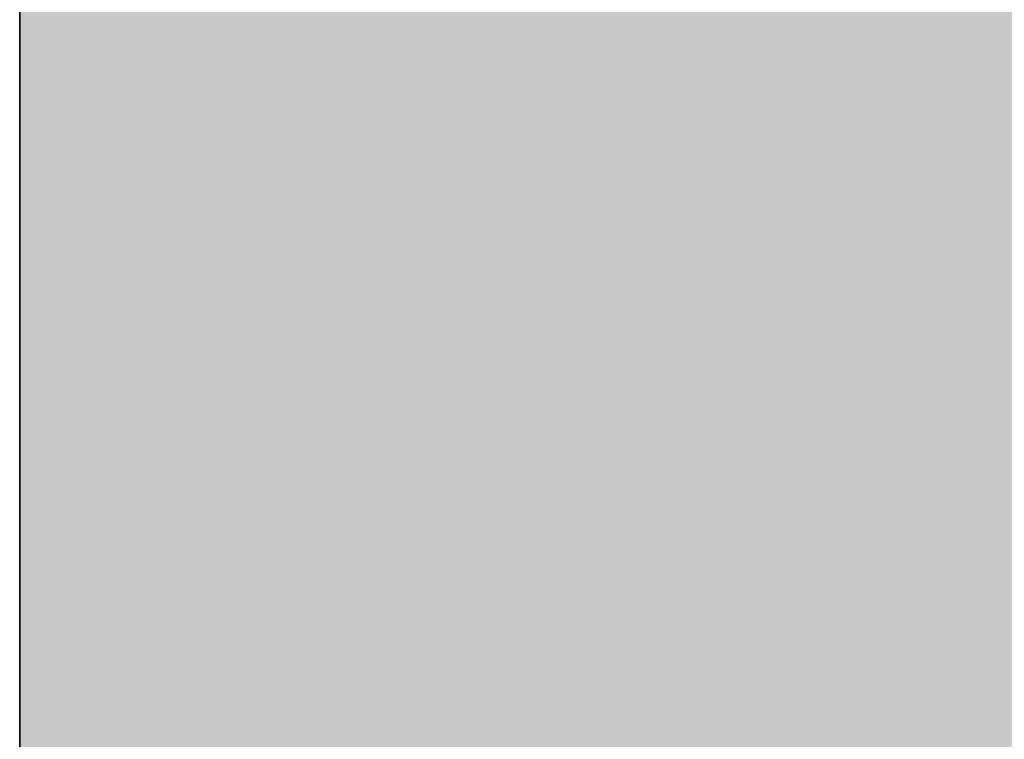
# Model space of a CAD drawing. Units: inches. Extents: x 2091 to 2899, y 967 to 2217.
# Tile 190 of 256: x 2203.1436 to 2203.18039, y 1152.27396 to 1152.30086. Entities that reach past the tile are written whole.
import ezdxf

# ---------------------------------------------------------------- set-up
doc = ezdxf.new("R2010")
doc.units = ezdxf.units.IN
doc.layers.add('A-WALL-PATT', color=141, linetype='Continuous', lineweight=13, true_color=0xadddf7)
doc.layers.add('C-PROP', color=7, linetype='Continuous', lineweight=35)

msp = doc.modelspace()

# ---------------------------------------------------------------- hatches: boundary and pattern name
at = {"layer": 'A-WALL-PATT'}
h = msp.add_hatch(color=256, dxfattribs=at)
h.dxf.hatch_style = 1
h.paths.add_polyline_path([(2803.143603, 2050.919059), (2203.143603, 2050.919059), (2203.143603, 1090.919059), (2803.143603, 1090.919059)])
h.paths.add_polyline_path([(2635.79885, 1147.540465), (2674.524052, 1147.540465, 0.376086), (2678.529665, 1152.880202), (2678.529665, 1159.556473, 0.333335), (2674.524319, 1163.561846), (2674.524319, 1163.56185), (2674.524319, 1192.93439), (2635.805971, 1192.93439), (2597.087622, 1192.93439), (2597.087622, 1163.561846, 0.333335), (2593.082276, 1159.556473), (2593.082276, 1152.880202, 0.376086), (2597.087889, 1147.540465)], flags=0)
h.paths.add_polyline_path([(2436.010433, 1278.240778, 0.000483), (2435.952643, 1278.215027, -0.001328), (2435.935625, 1278.111693, -0.001711), (2436.11644, 1278.040758, 0.002185)], flags=0)
h.paths.add_polyline_path([(2794.143603, 1143.419059), (2794.143603, 1347.419059), (2543.370171, 1347.419059), (2543.370171, 1351.919059), (2794.143603, 1351.919059), (2794.143603, 1392.713555), (2793.947398, 1392.713555), (2793.947398, 1473.5369), (2794.143603, 1473.5369), (2794.143603, 1531.919059), (2650.143603, 1531.919059), (2650.143603, 1536.419059), (2794.143603, 1536.419059), (2794.143603, 1692.419059), (2609.375609, 1692.419059), (2609.375609, 1644.419059), (2604.875609, 1644.419059), (2604.875609, 1744.919059), (2609.375609, 1744.919059), (2609.375609, 1696.919059), (2794.143603, 1696.919059), (2794.143603, 1780.919059), (2609.643603, 1780.919059), (2493.875609, 1780.919059), (2493.875609, 1785.419059), (2609.643603, 1785.419059), (2794.143603, 1785.419059), (2794.143603, 1847.938821), (2793.951222, 1847.938821), (2793.951222, 1928.762166), (2794.143603, 1928.762166), (2794.143603, 1941.419059), (2614.143603, 1941.419059), (2614.143603, 1821.419059), (2609.643603, 1821.419059), (2609.643603, 1941.419059), (2392.143603, 1941.419059), (2392.143603, 1819.919059), (2387.643603, 1819.919059), (2387.643603, 1941.419059), (2212.143603, 1941.419059), (2212.143603, 1783.919059), (2392.143603, 1783.919059), (2392.143603, 1780.919059), (2212.143603, 1780.919059), (2212.143603, 1629.419059), (2387.643603, 1629.419059), (2387.643603, 1744.919059), (2392.143603, 1744.919059), (2392.143603, 1627.919059), (2317.143603, 1627.919059), (2317.143603, 1551.419059), (2317.143603, 1536.419059), (2459.383591, 1536.419059), (2459.383591, 1602.39648), (2463.883591, 1602.39648), (2463.883591, 1531.919059), (2456.643603, 1531.919059), (2456.643603, 1529.919059), (2452.143603, 1529.919059), (2452.143603, 1531.919059), (2312.643603, 1531.919059), (2312.643603, 1551.419059), (2306.143603, 1551.419059), (2306.143603, 1555.919059), (2308.143603, 1555.919059), (2308.143603, 1551.419059), (2312.643603, 1551.419059), (2312.643603, 1627.919059), (2212.143603, 1627.919059), (2212.143603, 1555.919059), (2270.143603, 1555.919059), (2270.143603, 1551.419059), (2212.143603, 1551.419059), (2212.143603, 1351.919059), (2272.143603, 1351.919059), (2272.143603, 1347.419059), (2212.143603, 1347.419059), (2212.143603, 1275.419059), (2308.143603, 1275.419059), (2308.143603, 1351.919059), (2452.143603, 1351.919059), (2452.143603, 1493.919059), (2456.643603, 1493.919059), (2456.643603, 1347.419059), (2312.643603, 1347.419059), (2312.643603, 1270.919059), (2212.143603, 1270.919059), (2212.143603, 1099.919059), (2281.237523, 1099.919059), (2282.871041, 1110.913803), (2282.008341, 1116.996603), (2278.557741, 1121.420403), (2268.205641, 1128.056203), (2272.087641, 1128.056203), (2273.812941, 1131.927003), (2279.420341, 1134.691903), (2285.027841, 1135.244903), (2287.615841, 1137.456803), (2288.047141, 1138.009803), (2289.341141, 1140.774703), (2291.066541, 1139.668703), (2292.360541, 1135.244903), (2295.379841, 1136.903803), (2296.242541, 1135.797903), (2297.105241, 1133.033003), (2300.124641, 1138.009803), (2303.143941, 1138.009803), (2304.437941, 1135.797903), (2303.143941, 1133.586003), (2306.594641, 1134.691903), (2307.888741, 1133.033003), (2310.908041, 1135.244903), (2313.927441, 1134.138903), (2315.62686, 1132.427102), (2308.320041, 1117.549603), (2290.203841, 1109.807903), (2288.909841, 1103.172103), (2289.272309, 1099.919059), (2434.918227, 1099.919059), (2431.593227, 1124.788059), (2429.930227, 1169.553059), (2430.927185, 1240.519694), (2435.658926, 1238.186126), (2437.135227, 1196.554059), (2438.798227, 1143.973059), (2442.678227, 1111.998059), (2446.558227, 1099.919059), (2794.143603, 1099.919059), (2794.143603, 1138.919059), (2548.032447, 1138.919059), (2548.032447, 1143.419059), (2548.032447, 1148.819059), (2546.668457, 1148.031559), (2528.685692, 1179.178622, 0.256256), (2512.032447, 1148.819059), (2512.032447, 1143.419059), (2512.032447, 1138.919059), (2507.532447, 1138.919059), (2507.532447, 1143.419059), (2507.532447, 1148.819059, 0.256256), (2490.879202, 1179.178622), (2472.896437, 1148.031559), (2471.532447, 1148.819059), (2471.532447, 1143.419059), (2467.032447, 1143.419059), (2467.032447, 1269.945786, 0.039061), (2460.909987, 1273.580059), (2467.032447, 1273.580059), (2467.032447, 1286.325364, 0.014511), (2465.216194, 1286.761905), (2467.032447, 1287.052576), (2467.032447, 1323.419059), (2471.532447, 1323.419059), (2471.532447, 1148.819059), (2489.532447, 1179.995973), (2490.896437, 1179.208473), (2490.879202, 1179.178622, -0.256256), (2507.532447, 1148.819059), (2507.532447, 1143.419059), (2512.032447, 1143.419059), (2512.032447, 1148.819059, -0.256256), (2528.685692, 1179.178622), (2528.668457, 1179.208473), (2530.032447, 1179.995973), (2548.032447, 1148.819059), (2548.032447, 1143.419059)], flags=16)
h.paths.add_polyline_path([(2607.768546, 1200.945083), (2607.768546, 1265.030625), (2597.087622, 1281.052011), (2619.784585, 1281.052011), (2627.795278, 1337.12686), (2635.79885, 1337.12686), (2643.816663, 1337.12686), (2651.827356, 1281.052011), (2674.524319, 1281.052011), (2663.843395, 1265.030625), (2663.843395, 1200.945083), (2635.805971, 1200.945083)], flags=0)
edge = h.paths.add_edge_path(flags=0)
edge.add_ellipse((13303.896215, 1272.998725), major_axis=(-10595.31304, 0.000001), ratio=0.842303870086, start_angle=0.6282372191, end_angle=0.6465540999, ccw=False)
edge.add_ellipse((2711.70045, 1156.852678), major_axis=(2.219769, 0), ratio=0.84230387, start_angle=111.535244, end_angle=180.628237, ccw=False)
edge.add_ellipse((13303.156292, 1272.998725), major_axis=(-10593.026306, 0), ratio=0.842303869544, start_angle=0.5282714718, end_angle=0.6465540971, ccw=False)
edge.add_line((2710.764596, 1175.333295), (2710.129986, 1175.333295))
edge.add_ellipse((2710.129986, 1176.579775), major_axis=(1.479846, 0), ratio=0.84230387, start_angle=180, end_angle=270, ccw=False)
edge.add_line((2708.65014, 1176.579775), (2708.65014, 1200.782914))
edge.add_ellipse((2710.129986, 1200.782914), major_axis=(1.479846, 0), ratio=0.84230387, start_angle=90, end_angle=180, ccw=False)
edge.add_line((2710.129986, 1202.029394), (2710.465075, 1202.029394))
edge.add_ellipse((13303.156292, 1272.998725), major_axis=(-10593.026306, 0), ratio=0.842303869544, start_angle=-0.0902290886, end_angle=0.3838667788, ccw=False)
edge.add_ellipse((2710.129986, 1290.927031), major_axis=(-1.479846, 0), ratio=0.84230387, start_angle=0, end_angle=90, ccw=False)
edge.add_line((2708.65014, 1290.927031), (2708.65014, 1315.13017))
edge.add_ellipse((2710.129986, 1315.13017), major_axis=(-1.479846, 0), ratio=0.84230387, start_angle=-90, end_angle=0, ccw=False)
edge.add_line((2710.129986, 1316.37665), (2710.706314, 1316.37665))
edge.add_ellipse((3238.40172, 1296.289566), major_axis=(528.234, 0), ratio=0.8423038695, start_angle=176.34957241, end_angle=177.82004969, ccw=False)
edge.add_ellipse((2775.063043, 1071.450696), major_axis=(313.307761, 0), ratio=0.8423038695, start_angle=102.12596555, end_angle=103.78052899, ccw=False)
edge.add_ellipse((2775.063043, 1078.305698), major_axis=(-305.302891, 0), ratio=0.8423038695, start_angle=-79.790461, end_angle=-77.55537271, ccw=False)
edge.add_ellipse((2695.141767, 1541.975383), major_axis=(-250.960216, 0), ratio=0.8423038695, start_angle=99.25656601, end_angle=102.55493264)
edge.add_line((2741.410326, 1334.214255), (2747.132545, 1337.378477))
edge.add_ellipse((2747.538616, 1336.857478), major_axis=(-0.739923, 0), ratio=0.8423039, start_angle=270, end_angle=307.93313, ccw=False)
edge.add_ellipse((2747.538616, 1336.857478), major_axis=(-0.739923, 0), ratio=0.8423039, start_angle=232.06687, end_angle=270, ccw=False)
edge.add_line((2747.944687, 1337.378477), (2753.666906, 1334.214255))
edge.add_ellipse((2799.935466, 1541.975383), major_axis=(250.960216, 0), ratio=0.8423038695, start_angle=257.44506736, end_angle=260.74343399)
edge.add_ellipse((2720.014189, 1078.305698), major_axis=(305.302891, 0), ratio=0.8423038695, start_angle=77.55537271, end_angle=79.790461, ccw=False)
edge.add_ellipse((2720.014189, 1071.450696), major_axis=(-313.307761, 0), ratio=0.8423038695, start_angle=256.21947101, end_angle=257.87403445, ccw=False)
edge.add_ellipse((2256.675512, 1296.289566), major_axis=(-528.234, 0), ratio=0.8423038695, start_angle=182.17995031, end_angle=183.65042759, ccw=False)
edge.add_line((2784.370918, 1316.37665), (2784.947247, 1316.37665))
edge.add_ellipse((2784.947247, 1315.13017), major_axis=(1.479846, 0), ratio=0.84230387, start_angle=0, end_angle=90, ccw=False)
edge.add_line((2786.427093, 1315.13017), (2786.427093, 1290.927031))
edge.add_ellipse((2784.947247, 1290.927031), major_axis=(1.479846, 0), ratio=0.84230387, start_angle=270, end_angle=360, ccw=False)
edge.add_ellipse((-7808.07906, 1272.998725), major_axis=(10593.026306, 0), ratio=0.842303869544, start_angle=-0.3838667788, end_angle=0.0902290886, ccw=False)
edge.add_line((2784.612157, 1202.029394), (2784.947247, 1202.029394))
edge.add_ellipse((2784.947247, 1200.782914), major_axis=(1.479846, 0), ratio=0.84230387, start_angle=0, end_angle=90, ccw=False)
edge.add_line((2786.427093, 1200.782914), (2786.427093, 1176.579775))
edge.add_ellipse((2784.947247, 1176.579775), major_axis=(-1.479846, 0), ratio=0.84230387, start_angle=90, end_angle=180, ccw=False)
edge.add_line((2784.947247, 1175.333295), (2784.312636, 1175.333295))
edge.add_ellipse((-7808.07906, 1272.998725), major_axis=(10593.026306, 0), ratio=0.842303869544, start_angle=-0.6186431963, end_angle=-0.5282714718, ccw=False)
edge.add_ellipse((2783.376783, 1156.852678), major_axis=(-2.219769, 0), ratio=0.84230387, start_angle=179.371763, end_angle=248.464757, ccw=False)
edge.add_ellipse((-7808.818983, 1272.998725), major_axis=(-10595.31304, 0.000004), ratio=0.842303865762, start_angle=179.3534459226, end_angle=179.3717628034, ccw=False)
edge.add_ellipse((2780.297303, 1153.500793), major_axis=(-5.246426, 0), ratio=0.84230387, start_angle=90, end_angle=179.353446, ccw=False)
edge.add_line((2780.297303, 1149.081708), (2714.77993, 1149.081708))
edge.add_ellipse((2714.77993, 1153.500793), major_axis=(5.246426, 0), ratio=0.84230387, start_angle=180.646554, end_angle=270, ccw=False)
edge = h.paths.add_edge_path(flags=0)
edge.add_line((2718.187367, 1151.007833), (2718.187367, 1170.472364))
edge.add_ellipse((2721.14706, 1170.472364), major_axis=(-2.959692, 0), ratio=0.84230387, start_angle=-90, end_angle=0, ccw=False)
edge.add_line((2721.14706, 1172.965324), (2773.930173, 1172.965324))
edge.add_ellipse((2773.930173, 1170.472364), major_axis=(-2.959692, 0), ratio=0.84230387, start_angle=180, end_angle=270, ccw=False)
edge.add_line((2776.889865, 1170.472364), (2776.889865, 1151.007833))
edge.add_line((2776.889865, 1151.007833), (2718.187367, 1151.007833))
edge = h.paths.add_edge_path(flags=0)
edge.add_line((2718.187367, 1180.23415), (2718.187367, 1199.057834))
edge.add_ellipse((2747.538616, 1320.39864), major_axis=(147.017924, 0), ratio=0.8423038695, start_angle=256.40186531, end_angle=283.59813469)
edge.add_line((2776.889865, 1199.057834), (2776.889865, 1180.23415))
edge.add_ellipse((2747.538616, 1301.574956), major_axis=(147.017924, 0), ratio=0.8423038695, start_angle=256.40186531, end_angle=283.59813469, ccw=False)
edge = h.paths.add_edge_path(flags=0)
edge.add_ellipse((13303.156292, 1272.998725), major_axis=(-10591.54646, 0), ratio=0.842303869555, start_angle=0.0555943135, end_angle=0.3777641939, ccw=False)
edge.add_line((2711.616859, 1262.72171), (2715.667408, 1249.495396))
edge.add_ellipse((6413.891963, 1241.691919), major_axis=(-3698.236159, 0), ratio=0.84230386955, start_angle=-0.120897369, end_angle=0.364076349)
edge.add_line((2715.761038, 1218.192455), (2711.934307, 1203.167361))
edge = h.paths.add_edge_path(flags=0)
edge.add_line((2718.187367, 1251.074566), (2716.002485, 1267.450435))
edge.add_ellipse((2742.151175, 1202.18954), major_axis=(81.772585, 0), ratio=0.84230387, start_angle=94.27742096, end_angle=111.8349538, ccw=False)
edge.add_line((2737.009748, 1270.930626), (2758.067484, 1270.930626))
edge.add_ellipse((2752.926058, 1202.18954), major_axis=(81.772585, 0), ratio=0.84230387, start_angle=68.1650462, end_angle=85.72257904, ccw=False)
edge.add_line((2779.074747, 1267.450435), (2776.889865, 1251.074566))
edge.add_ellipse((2750.338059, 1187.885356), major_axis=(79.579664, 0), ratio=0.84230387, start_angle=67.20808512, end_angle=85.1299304)
edge.add_line((2756.034656, 1254.743656), (2739.042576, 1254.743656))
edge.add_ellipse((2744.739174, 1187.885356), major_axis=(79.579664, 0), ratio=0.84230387, start_angle=94.8700696, end_angle=112.79191488)
edge = h.paths.add_edge_path(flags=0)
edge.add_line((2783.142926, 1203.167361), (2779.316194, 1218.192455))
edge.add_ellipse((-918.81473, 1241.691919), major_axis=(3698.236159, 0), ratio=0.84230386955, start_angle=-0.364076349, end_angle=0.120897369)
edge.add_line((2779.409825, 1249.495396), (2783.460373, 1262.72171))
edge.add_ellipse((-7808.07906, 1272.998725), major_axis=(-10591.54646, 0), ratio=0.84230386954, start_angle=179.6222358061, end_angle=179.9444056865, ccw=False)
edge = h.paths.add_edge_path(flags=0)
edge.add_ellipse((2734.200892, 1286.69044), major_axis=(-0.356609, 6.340078), ratio=0.60383358, start_angle=89.0020143, end_angle=253.657408, ccw=False)
edge.add_line((2730.369001, 1286.541806), (2730.369001, 1301.35198))
edge.add_line((2730.369001, 1301.35198), (2735.913311, 1305.214803))
edge.add_ellipse((2736.384917, 1304.734561), major_axis=(0.739923, 0), ratio=0.8423039, start_angle=90, end_angle=134.480211, ccw=False)
edge.add_line((2736.384917, 1305.357801), (2738.032783, 1305.357801))
edge.add_line((2738.032783, 1305.357801), (2738.032783, 1307.707927))
edge.add_ellipse((2794.201642, 1307.707927), major_axis=(56.168859, 0), ratio=0.84230387, start_angle=150.5614304, end_angle=180, ccw=False)
edge.add_ellipse((2700.875591, 1307.707927), major_axis=(-56.168859, 0), ratio=0.84230387, start_angle=180, end_angle=209.4385696, ccw=False)
edge.add_line((2757.04445, 1307.707927), (2757.04445, 1305.357801))
edge.add_line((2757.04445, 1305.357801), (2758.692316, 1305.357801))
edge.add_ellipse((2758.692316, 1304.734561), major_axis=(-0.739923, 0), ratio=0.8423039, start_angle=225.519789, end_angle=270, ccw=False)
edge.add_line((2759.163922, 1305.214803), (2764.708231, 1301.35198))
edge.add_line((2764.708231, 1301.35198), (2764.708231, 1286.541806))
edge.add_ellipse((2760.87634, 1286.69044), major_axis=(0.356609, 6.340078), ratio=0.60383358, start_angle=106.342592, end_angle=270.9979857, ccw=False)
edge.add_line((2757.04445, 1285.79709), (2757.04445, 1307.707927))
edge.add_ellipse((2700.875591, 1307.707927), major_axis=(-56.168859, 0), ratio=0.84230387, start_angle=180, end_angle=209.4385696)
edge.add_ellipse((2794.201642, 1307.707927), major_axis=(56.168859, 0), ratio=0.84230387, start_angle=150.5614304, end_angle=180)
edge.add_line((2738.032783, 1307.707927), (2738.032783, 1285.79709))
h.paths.add_polyline_path([(2417.812273, 1104.449704), (2413.492273, 1102.529704), (2410.612273, 1103.969704), (2409.172273, 1106.369704), (2407.252273, 1107.329704), (2406.292273, 1109.729704), (2405.332273, 1114.049704), (2405.332273, 1117.889704), (2406.292273, 1120.129704), (2407.252273, 1119.809704), (2408.848322, 1118.327658), (2410.173945, 1119.42417), (2410.211273, 1120.405704), (2411.040731, 1121.419054), (2410.699273, 1119.858704), (2410.173945, 1119.42417), (2410.088452, 1117.176109), (2411.132836, 1116.206324), (2413.972273, 1119.329704), (2416.852273, 1120.769704), (2416.869721, 1120.798784), (2417.035071, 1119.405116), (2417.896213, 1118.143384), (2418.292273, 1118.369704), (2419.544447, 1120.039269), (2419.360915, 1118.387487), (2419.032108, 1119.356151), (2418.398939, 1118.511926), (2419.252273, 1114.529704), (2418.794091, 1107.198795)], flags=0)
h.paths.add_polyline_path([(2508.870171, 1347.419059), (2508.370171, 1347.419059), (2508.370171, 1351.919059), (2508.870171, 1351.919059)], flags=0)
h.paths.add_polyline_path([(2473.370171, 1347.419059), (2472.370171, 1347.419059), (2467.870171, 1347.419059), (2467.870171, 1455.419059), (2472.370171, 1455.419059), (2472.370171, 1352.419059), (2473.370171, 1352.419059)], flags=0)
h.paths.add_polyline_path([(2352.106244, 1217.446197), (2349.226244, 1218.886197), (2347.786244, 1221.286197), (2345.866244, 1222.246197), (2344.906244, 1224.646197), (2343.946244, 1228.966197), (2343.946244, 1232.806197), (2344.906244, 1235.046197), (2345.866244, 1234.726197), (2347.462293, 1233.244152), (2348.787916, 1234.340663), (2348.825244, 1235.322197), (2349.654702, 1236.335547), (2349.313244, 1234.775197), (2348.787916, 1234.340663), (2348.702423, 1232.092603), (2349.746807, 1231.122817), (2352.586244, 1234.246197), (2355.466244, 1235.686197), (2355.483692, 1235.715277), (2355.649043, 1234.321609), (2356.510185, 1233.059877), (2356.906244, 1233.286197), (2358.158418, 1234.955762), (2357.974887, 1233.30398), (2357.646079, 1234.272644), (2357.012911, 1233.428419), (2357.866244, 1229.446197), (2357.408062, 1222.115288), (2356.426244, 1219.366197)], flags=0)
h.paths.add_polyline_path([(2348.2968, 1112.22442), (2347.0138, 1112.31042), (2345.5298, 1114.12742), (2345.7318, 1115.85842), (2346.8118, 1116.98242), (2346.8118, 1114.64642), (2345.8668, 1114.21442), (2346.8798, 1114.30042)], flags=0)
h.paths.add_polyline_path([(2347.0138, 1110.92642), (2346.2718, 1110.49342), (2346.6098, 1111.18642)], flags=0)
h.paths.add_polyline_path([(2345.8668, 1118.19442), (2345.5298, 1117.32942), (2343.7078, 1118.02142), (2344.3828, 1118.62642)], flags=0)
h.paths.add_polyline_path([(2346.6768, 1109.28242), (2346.0698, 1108.07142), (2345.8668, 1110.06142)], flags=0)
h.paths.add_polyline_path([(2345.0568, 1119.75142), (2343.6398, 1119.75142), (2343.9778, 1121.13542)], flags=0)
h.paths.add_polyline_path([(2345.2598, 1116.55042), (2345.1248, 1115.85842), (2344.9218, 1115.68542), (2344.7198, 1116.37742)], flags=0)
h.paths.add_polyline_path([(2345.6648, 1112.31042), (2345.4618, 1111.53242), (2344.0448, 1111.96442), (2344.6518, 1112.57042)], flags=0)
h.paths.add_polyline_path([(2345.1918, 1113.34942), (2344.4498, 1113.86842), (2344.7198, 1114.38742)], flags=0)
h.paths.add_polyline_path([(2344.6518, 1116.80942), (2344.1798, 1115.68542), (2344.6518, 1115.33942), (2343.9098, 1114.90642), (2343.0328, 1115.94442), (2343.6398, 1116.46342)], flags=0)
h.paths.add_polyline_path([(2345.8668, 1106.68642), (2344.9898, 1105.56242), (2344.5168, 1106.60042)], flags=0)
h.paths.add_polyline_path([(2344.8548, 1110.06142), (2344.5168, 1109.28242), (2344.1128, 1109.71542)], flags=0)
h.paths.add_polyline_path([(2344.0448, 1113.52242), (2343.4378, 1113.08942), (2342.7628, 1113.95442)], flags=0)
h.paths.add_polyline_path([(2344.3148, 1111.01242), (2342.9648, 1110.32042), (2342.9648, 1111.09942)], flags=0)
h.paths.add_polyline_path([(2345.1248, 1104.69742), (2344.5848, 1103.74542), (2344.4498, 1104.26442)], flags=0)
h.paths.add_polyline_path([(2342.8298, 1121.22242), (2341.7498, 1120.53042), (2340.5358, 1121.04942), (2340.1308, 1121.82842), (2340.6708, 1122.95242), (2341.1428, 1121.82842), (2341.6148, 1122.00142)], flags=0)
h.paths.add_polyline_path([(2342.9648, 1119.75142), (2343.0328, 1118.45342), (2342.0878, 1118.02142), (2342.0198, 1119.49142)], flags=0)
h.paths.add_polyline_path([(2342.6948, 1116.89642), (2341.9528, 1116.63642), (2342.0198, 1117.32942)], flags=0)
h.paths.add_polyline_path([(2343.0328, 1112.22442), (2342.0198, 1111.79142), (2341.5478, 1112.22442), (2342.3578, 1113.34942)], flags=0)
h.paths.add_polyline_path([(2343.7748, 1104.43742), (2342.6278, 1102.88042), (2342.6948, 1104.61042), (2343.4378, 1105.12942)], flags=0)
h.paths.add_polyline_path([(2342.0198, 1115.07942), (2340.8058, 1115.51242), (2340.9408, 1116.37742)], flags=0)
h.paths.add_polyline_path([(2341.4808, 1120.09742), (2341.4808, 1119.40542), (2341.0758, 1119.57842), (2341.1428, 1120.09742)], flags=0)
h.paths.add_polyline_path([(2341.8178, 1114.47342), (2340.9408, 1113.08942), (2340.8058, 1114.56042)], flags=0)
h.paths.add_polyline_path([(2341.1428, 1118.54042), (2340.9408, 1116.98242), (2339.0508, 1117.67542), (2339.0508, 1118.62642)], flags=0)
h.paths.add_polyline_path([(2342.6948, 1101.66842), (2341.9528, 1101.84142), (2342.5598, 1102.36142)], flags=0)
h.paths.add_polyline_path([(2340.3328, 1119.66542), (2338.4438, 1119.57842), (2337.9038, 1120.35742), (2339.6578, 1120.61642)], flags=0)
h.paths.add_polyline_path([(2340.3328, 1115.33942), (2340.0628, 1113.69542), (2339.3878, 1115.33942)], flags=0)
h.paths.add_polyline_path([(2341.8178, 1103.83142), (2341.5478, 1102.88042), (2341.1428, 1103.65842)], flags=0)
h.paths.add_polyline_path([(2339.0508, 1122.86642), (2337.2958, 1121.82842), (2337.0938, 1123.12542), (2337.7688, 1123.81842)], flags=0)
h.paths.add_polyline_path([(2339.1178, 1121.74142), (2338.8478, 1121.22242), (2338.1738, 1121.04942), (2338.3758, 1121.56842)], flags=0)
h.paths.add_polyline_path([(2339.1858, 1119.31942), (2338.6458, 1118.71342), (2338.2408, 1118.10742), (2338.2408, 1118.88642)], flags=0)
h.paths.add_polyline_path([(2341.1428, 1101.92842), (2340.6028, 1101.23642), (2340.0628, 1101.84142), (2340.6028, 1102.36142)], flags=0)
h.paths.add_polyline_path([(2337.6338, 1117.76142), (2336.6208, 1118.28042), (2337.2958, 1118.97242)], flags=0)
h.paths.add_polyline_path([(2336.8238, 1119.57842), (2334.7988, 1118.97242), (2335.2038, 1120.35742), (2336.5538, 1120.87642)], flags=0)
h.paths.add_polyline_path([(2339.1178, 1100.45742), (2337.3638, 1100.54342), (2336.7558, 1101.23642)], flags=0)
h.paths.add_polyline_path([(2336.3508, 1122.43342), (2336.0138, 1121.91442), (2334.9338, 1122.43342), (2334.5288, 1123.47142), (2335.7438, 1122.77942)], flags=0)
h.paths.add_polyline_path([(2334.7318, 1120.87642), (2334.2588, 1120.35742), (2334.0568, 1120.78942), (2334.5968, 1121.30842)], flags=0)
h.paths.add_polyline_path([(2334.4618, 1122.17442), (2332.5718, 1121.30842), (2331.3568, 1122.17442), (2332.0998, 1122.86642)], flags=0)
h.paths.add_polyline_path([(2334.2588, 1118.54042), (2333.3818, 1118.45342), (2333.6518, 1119.31942)], flags=0)
h.paths.add_polyline_path([(2335.5418, 1102.27442), (2334.1918, 1102.62042), (2335.2718, 1103.31242)], flags=0)
h.paths.add_polyline_path([(2332.7068, 1119.66542), (2331.6948, 1120.44342), (2332.5048, 1120.78942)], flags=0)
h.paths.add_polyline_path([(2334.7318, 1101.14942), (2333.5168, 1101.58242), (2333.9888, 1101.75542)], flags=0)
h.paths.add_polyline_path([(2332.6398, 1116.63642), (2331.0868, 1116.29042), (2331.9648, 1118.19442)], flags=0)
h.paths.add_polyline_path([(2330.7498, 1121.56842), (2330.2768, 1120.27042), (2328.5228, 1119.31942), (2328.9948, 1121.04942)], flags=0)
h.paths.add_polyline_path([(2330.7498, 1118.62642), (2330.0078, 1117.50242), (2329.8728, 1118.02142)], flags=0)
h.paths.add_polyline_path([(2332.0998, 1102.36142), (2330.5468, 1102.01442), (2331.6948, 1102.96642)], flags=0)
h.paths.add_polyline_path([(2329.5348, 1113.60842), (2329.0628, 1112.31042), (2328.5898, 1113.34942)], flags=0)
h.paths.add_polyline_path([(2328.3878, 1117.84842), (2327.5098, 1116.55042), (2327.1728, 1117.76142)], flags=0)
h.paths.add_polyline_path([(2329.7378, 1106.51342), (2329.5348, 1105.30242), (2328.2528, 1106.08142)], flags=0)
h.paths.add_polyline_path([(2328.6578, 1114.38742), (2328.0498, 1114.12742), (2328.3198, 1114.90642)], flags=0)
h.paths.add_polyline_path([(2328.3198, 1112.22442), (2327.1058, 1112.13742), (2326.7008, 1112.65642)], flags=0)
h.paths.add_polyline_path([(2326.9028, 1115.25242), (2326.7008, 1114.12742), (2325.2158, 1113.60842), (2326.0928, 1115.33942)], flags=0)
h.paths.add_polyline_path([(2326.6328, 1108.33042), (2326.0928, 1107.37942), (2325.8908, 1108.50342), (2326.4978, 1109.10942)], flags=0)
h.paths.add_polyline_path([(2615.143603, 1531.919059), (2609.643603, 1531.919059), (2609.643603, 1620.419059), (2614.143603, 1620.419059), (2614.143603, 1536.419059), (2615.143603, 1536.419059)], flags=0)
h.paths.add_polyline_path([(2545.143603, 1563.419059), (2464.143603, 1563.419059), (2464.143603, 1632.419059), (2509.143603, 1632.419059), (2509.143603, 1627.919059), (2509.143603, 1603.919059), (2468.643603, 1603.919059), (2468.643603, 1567.919059), (2540.643603, 1567.919059), (2540.643603, 1591.919059), (2545.143603, 1591.919059)], flags=0)
h.paths.add_polyline_path([(2388.969048, 1549.985735), (2357.434181, 1549.985735), (2357.434181, 1623.360778), (2399.362777, 1623.360778), (2435.689465, 1623.360778), (2435.592547, 1602.559273), (2435.592547, 1602.39648), (2388.969048, 1602.39648)], flags=0)
h.paths.add_polyline_path([(2388.880628, 1555.809151), (2374.904429, 1555.809151), (2374.904429, 1600.571564), (2374.904429, 1615.457645), (2406.350877, 1615.457645), (2406.350877, 1618.939431), (2412.174293, 1615.457645), (2406.350877, 1611.97586), (2406.350877, 1615.457645), (2388.880628, 1615.457645)], flags=0)
h.paths.add_polyline_path([(2568.875609, 1644.419059), (2453.375609, 1644.419059), (2453.375609, 1785.419059), (2457.875609, 1785.419059), (2457.875609, 1648.919059), (2568.875609, 1648.919059)], flags=0)
h.paths.add_polyline_path([(2212.143603, 1945.919059), (2212.143603, 2041.919059), (2794.143603, 2041.919059), (2794.143603, 1945.919059)], flags=16)
h.paths.add_polyline_path([(2271.082728, 1964.317238), (2776.852968, 1964.317238), (2776.852968, 2037.169623), (2271.082728, 2037.169623)], flags=8)
h.paths.add_polyline_path([(2380.649285, 1536.824144), (2461.040809, 1536.824144), (2461.040809, 1554.652587), (2380.649285, 1554.652587)], flags=8)
h.paths.add_polyline_path([(2240.755709, 1609.725451), (2309.185829, 1609.725451), (2309.185829, 1617.698204), (2240.755709, 1617.698204)], flags=8)
h.paths.add_polyline_path([(2212.677255, 1313.504102), (2282.59152, 1313.504102), (2282.59152, 1322.745239), (2212.677255, 1322.745239)], flags=8)
h.paths.add_polyline_path([(2457.111976, 1114.778574), (2558.481581, 1114.778574), (2558.481581, 1142.219682), (2457.111976, 1142.219682)], flags=8)
h.paths.add_polyline_path([(2473.442337, 1273.010067), (2604.641226, 1273.010067), (2604.641226, 1318.346935), (2473.442337, 1318.346935)], flags=8)
h.paths.add_polyline_path([(2638.876302, 1626.977432), (2684.250367, 1627.976738), (2684.038483, 1637.597494), (2638.664417, 1636.598188)], flags=8)
h.paths.add_polyline_path([(2537.590554, 1453.793447), (2628.389547, 1453.793447), (2628.389547, 1475.344811), (2537.590554, 1475.344811)], flags=8)
h.paths.add_polyline_path([(2504.137638, 1714.632397), (2554.647187, 1714.632397), (2554.647187, 1730.237712), (2504.137638, 1730.237712)], flags=8)
h.paths.add_polyline_path([(2487.501181, 1575.651872), (2535.097121, 1575.651872), (2535.097121, 1598.377646), (2487.501181, 1598.377646)], flags=8)
h.paths.add_polyline_path([(2709.0994, 1735.710278), (2740.016601, 1735.710278), (2740.016601, 1749.937641), (2709.0994, 1749.937641)], flags=8)
h.paths.add_polyline_path([(2442.438424, 1792.171657), (2564.728835, 1792.171657), (2564.728835, 1842.000163), (2442.438424, 1842.000163)], flags=8)
h.paths.add_polyline_path([(2655.815801, 1809.644076), (2789.520142, 1806.693796), (2790.084977, 1832.291638), (2656.380635, 1835.241918)], flags=8)
h.paths.add_polyline_path([(2234.842697, 1797.720143), (2368.592851, 1794.768852), (2369.160718, 1820.504132), (2235.410564, 1823.455423)], flags=8)
h.paths.add_polyline_path([(2245.138466, 1644.006335), (2398.427733, 1640.6239), (2398.994842, 1666.32482), (2245.705575, 1669.707255)], flags=8)
h.paths.add_polyline_path([(2306.142847, 1431.168519), (2413.768314, 1428.793687), (2414.333148, 1454.391529), (2306.707682, 1456.76636)], flags=8)
h.paths.add_polyline_path([(2306.834582, 1458.233145), (2393.380484, 1456.323449), (2393.932808, 1481.354358), (2307.386907, 1483.264054)], flags=8)

# ---------------------------------------------------------------- linework, layer by layer
at = {"layer": 'C-PROP'}
msp.add_lwpolyline([(2203.143603, 2050.919059), (2803.143603, 2050.919059), (2803.143603, 1090.919059), (2203.143603, 1090.919059)], close=True, dxfattribs=at)

doc.saveas('drawing.dxf')
